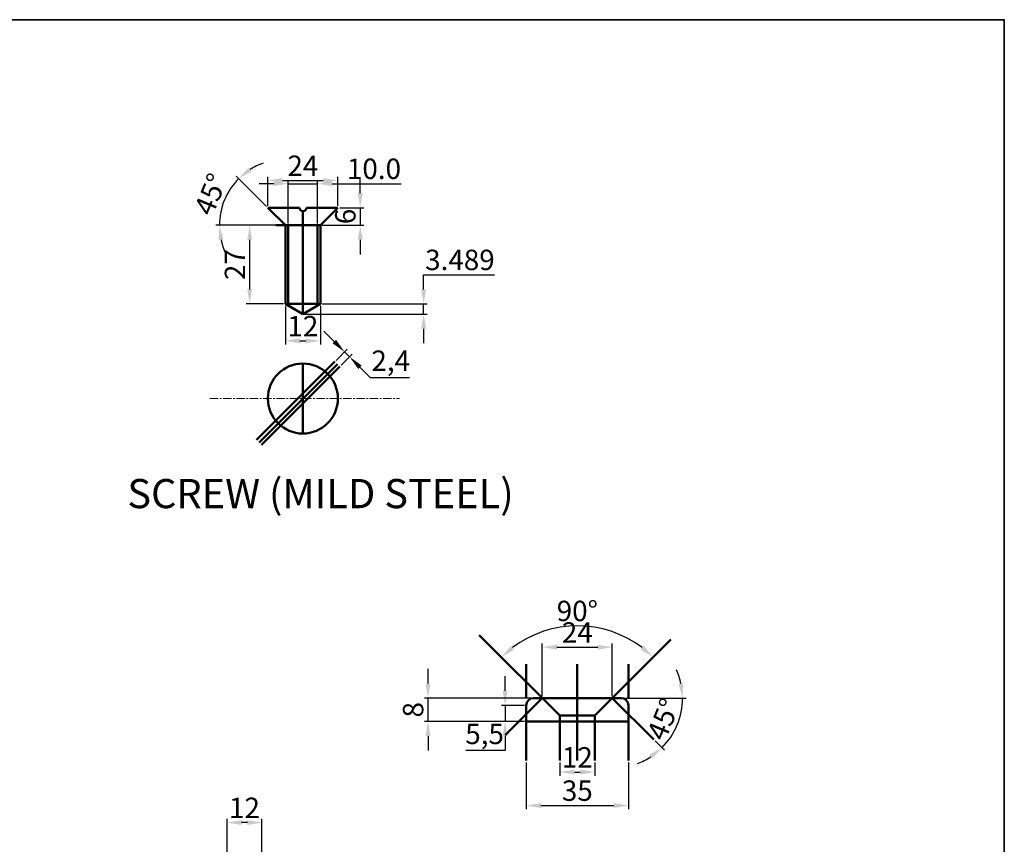
# Model space of a CAD drawing. Units: millimetres. Extents: x 4274 to 5106, y 2129 to 2785.
# Tile 4 of 4: x 4740 to 5077, y 2502 to 2785. Entities that reach past the tile are written whole.
import ezdxf

# ---------------------------------------------------------------- set-up
doc = ezdxf.new("R2010")
doc.units = ezdxf.units.MM
doc.header["$LTSCALE"] = 0.3
doc.linetypes.add('CENTER', pattern=[50.8, 31.75, -6.35, 6.35, -6.35])
for name, color, linetype, lineweight in [('M-CNTR', 1, 'CENTER', 18), ('M-DIMS', 2, 'Continuous', 25), ('M-OUTL', 7, 'Continuous', 50), ('M-TEXT', 3, 'Continuous', 25), ('M-TTLB', 7, 'Continuous', 35)]:
    doc.layers.add(name, color=color, linetype=linetype, lineweight=lineweight)
doc.styles.get("Standard").update_dxf_attribs({"font": 'arial.ttf'})
doc.dimstyles.new('ISO-25', dxfattribs={"dimtxt": 7, "dimasz": 5, "dimexe": 1.25, "dimexo": 0.625, "dimtad": 1, "dimtoh": 1, "dimtxsty": 'Standard', "dimcen": 2.5, "dimadec": 0, "dimazin": 0, "dimtfac": 1, "dimtmove": 0, "dimatfit": 3, "dimfxl": 1, "dimarcsym": 0})

# ---------------------------------------------------------------- blocks, each defined once
blk = doc.blocks.new('*D24')
at = {"layer": 'Defpoints', "color": 0, "ltscale": 0.3, "transparency": 16777216}
for p in [(4847.91, 2667.9), (4852.95, 2669.55), (4849.6, 2666.2)]:
    blk.add_point(p, dxfattribs=at)
at = {"layer": 'M-DIMS', "color": 0, "lineweight": -2, "ltscale": 0.3, "transparency": 16777216}
for p, q in [((4847.72, 2674.78), (4844.18, 2678.31)), ((4848.35, 2668.34), (4852.14, 2672.13)), ((4851.25, 2671.24), (4852.95, 2669.55)), ((4850.04, 2666.64), (4853.83, 2670.43)), ((4856.48, 2666.01), (4860.02, 2662.48)), ((4860.02, 2662.48), (4873.48, 2662.48))]:
    blk.add_line(p, q, dxfattribs=at)
at = {"layer": 'M-DIMS', "color": 0, "ltscale": 0.3, "transparency": 16777216}
for points in [[(4848.31, 2675.37), (4847.13, 2674.19), (4851.25, 2671.24)], [(4857.07, 2666.6), (4855.89, 2665.42), (4852.95, 2669.55)]]:
    blk.add_solid(points, dxfattribs=at)
at = {"layer": 'M-DIMS', "color": 0, "ltscale": 0.3, "transparency": 16777216, "insert": (4867.06, 2667.31), "char_height": 7, "attachment_point": 5}
blk.add_mtext('2,4', dxfattribs=at)
blk = doc.blocks.new('*D25')
at = {"layer": 'Defpoints', "color": 0, "ltscale": 0.3, "transparency": 16777216}
for p in [(4848.94, 2720.68), (4842.94, 2714.68), (4856.6, 2714.68)]:
    blk.add_point(p, dxfattribs=at)
at = {"layer": 'M-DIMS', "color": 0, "lineweight": -2, "ltscale": 0.3, "transparency": 16777216}
for p, q in [((4856.6, 2725.68), (4856.6, 2730.68)), ((4849.57, 2720.68), (4857.85, 2720.68)), ((4856.6, 2720.68), (4856.6, 2714.68)), ((4843.57, 2714.68), (4857.85, 2714.68)), ((4856.6, 2709.68), (4856.6, 2704.68))]:
    blk.add_line(p, q, dxfattribs=at)
at = {"layer": 'M-DIMS', "color": 0, "ltscale": 0.3, "transparency": 16777216}
for points in [[(4855.77, 2725.68), (4857.44, 2725.68), (4856.6, 2720.68)], [(4855.77, 2709.68), (4857.44, 2709.68), (4856.6, 2714.68)]]:
    blk.add_solid(points, dxfattribs=at)
at = {"layer": 'M-DIMS', "color": 0, "ltscale": 0.3, "transparency": 16777216, "insert": (4852.4, 2717.68), "char_height": 7, "attachment_point": 5, "rotation": 90}
blk.add_mtext('6', dxfattribs=at)
blk = doc.blocks.new('*D26')
at = {"layer": 'Defpoints', "color": 0, "ltscale": 0.3, "transparency": 16777216}
for p in [(4830.94, 2714.68), (4818.69, 2687.68), (4830.94, 2687.68)]:
    blk.add_point(p, dxfattribs=at)
at = {"layer": 'M-DIMS', "color": 0, "lineweight": -2, "ltscale": 0.3, "transparency": 16777216}
for p, q in [((4830.32, 2714.68), (4817.44, 2714.68)), ((4818.69, 2709.68), (4818.69, 2692.68)), ((4830.32, 2687.68), (4817.44, 2687.68))]:
    blk.add_line(p, q, dxfattribs=at)
at = {"layer": 'M-DIMS', "color": 0, "ltscale": 0.3, "transparency": 16777216}
for points in [[(4817.86, 2709.68), (4819.53, 2709.68), (4818.69, 2714.68)], [(4817.86, 2692.68), (4819.53, 2692.68), (4818.69, 2687.68)]]:
    blk.add_solid(points, dxfattribs=at)
at = {"layer": 'M-DIMS', "color": 0, "ltscale": 0.3, "transparency": 16777216, "insert": (4814.55, 2701.18), "char_height": 7, "attachment_point": 5, "rotation": 90}
blk.add_mtext('27', dxfattribs=at)
blk = doc.blocks.new('*D27')
at = {"layer": 'Defpoints', "color": 0, "ltscale": 0.3, "transparency": 16777216}
for p in [(4848.94, 2730.03), (4824.94, 2720.68), (4848.94, 2720.68)]:
    blk.add_point(p, dxfattribs=at)
at = {"layer": 'M-DIMS', "color": 0, "lineweight": -2, "ltscale": 0.3, "transparency": 16777216}
for p, q in [((4824.94, 2721.3), (4824.94, 2731.28)), ((4829.94, 2730.03), (4843.94, 2730.03)), ((4848.94, 2721.3), (4848.94, 2731.28))]:
    blk.add_line(p, q, dxfattribs=at)
at = {"layer": 'M-DIMS', "color": 0, "ltscale": 0.3, "transparency": 16777216}
for points in [[(4829.94, 2730.87), (4829.94, 2729.2), (4824.94, 2730.03)], [(4843.94, 2730.87), (4843.94, 2729.2), (4848.94, 2730.03)]]:
    blk.add_solid(points, dxfattribs=at)
at = {"layer": 'M-DIMS', "color": 0, "ltscale": 0.3, "transparency": 16777216, "insert": (4836.94, 2734.17), "char_height": 7, "attachment_point": 5}
blk.add_mtext('24', dxfattribs=at)
blk = doc.blocks.new('*D28')
at = {"layer": 'Defpoints', "color": 0, "ltscale": 0.3, "transparency": 16777216}
for p in [(4811.35, 2725.99), (4824.94, 2720.68), (4827.61, 2714.68), (4830.94, 2714.68), (4830.94, 2714.68)]:
    blk.add_point(p, dxfattribs=at)
at = {"layer": 'M-DIMS', "color": 0, "lineweight": -2, "ltscale": 0.3, "transparency": 16777216}
for p, q in [((4824.5, 2721.12), (4814.06, 2731.56)), ((4826.99, 2714.68), (4807.07, 2714.68))]:
    blk.add_line(p, q, dxfattribs=at)
for start, end in [(109.6287, 122.3144), (135, 180), (192.6856, 205.3713)]:
    blk.add_arc((4830.94, 2714.68), 22.63, start, end, dxfattribs=at)
at = {"layer": 'M-DIMS', "color": 0, "ltscale": 0.3, "transparency": 16777216}
for points in [[(4819.37, 2733.15), (4818.33, 2734.45), (4814.94, 2730.68)], [(4808.04, 2709.62), (4809.7, 2709.8), (4808.32, 2714.68)]]:
    blk.add_solid(points, dxfattribs=at)
at = {"layer": 'M-DIMS', "color": 0, "ltscale": 0.3, "transparency": 16777216, "insert": (4806.17, 2724.94), "char_height": 7, "attachment_point": 5, "rotation": 67.5}
blk.add_mtext('45°', dxfattribs=at)
blk = doc.blocks.new('*D29')
at = {"layer": 'Defpoints', "color": 0, "ltscale": 0.3, "transparency": 16777216}
for p in [(4830.94, 2687.68), (4842.94, 2687.68), (4842.94, 2675.03)]:
    blk.add_point(p, dxfattribs=at)
at = {"layer": 'M-DIMS', "color": 0, "lineweight": -2, "ltscale": 0.3, "transparency": 16777216}
for p, q in [((4830.94, 2687.05), (4830.94, 2673.78)), ((4842.94, 2687.05), (4842.94, 2673.78)), ((4835.94, 2675.03), (4837.94, 2675.03))]:
    blk.add_line(p, q, dxfattribs=at)
at = {"layer": 'M-DIMS', "color": 0, "ltscale": 0.3, "transparency": 16777216}
for points in [[(4835.94, 2675.87), (4835.94, 2674.2), (4830.94, 2675.03)], [(4837.94, 2675.87), (4837.94, 2674.2), (4842.94, 2675.03)]]:
    blk.add_solid(points, dxfattribs=at)
at = {"layer": 'M-DIMS', "color": 0, "ltscale": 0.3, "transparency": 16777216, "insert": (4836.94, 2679.17), "char_height": 7, "attachment_point": 5}
blk.add_mtext('12', dxfattribs=at)
blk = doc.blocks.new('*D34')
at = {"layer": 'Defpoints', "color": 0, "ltscale": 0.3, "transparency": 16777216}
for p in [(4810.92, 2509.83), (4810.92, 2495.1), (4822.92, 2495.1)]:
    blk.add_point(p, dxfattribs=at)
at = {"layer": 'M-DIMS', "color": 0, "lineweight": -2, "ltscale": 0.3, "transparency": 16777216}
for p, q in [((4810.92, 2495.72), (4810.92, 2511.08)), ((4817.92, 2509.83), (4815.92, 2509.83)), ((4822.92, 2495.72), (4822.92, 2511.08))]:
    blk.add_line(p, q, dxfattribs=at)
at = {"layer": 'M-DIMS', "color": 0, "ltscale": 0.3, "transparency": 16777216}
for points in [[(4815.92, 2510.66), (4815.92, 2508.99), (4810.92, 2509.83)], [(4817.92, 2510.66), (4817.92, 2508.99), (4822.92, 2509.83)]]:
    blk.add_solid(points, dxfattribs=at)
at = {"layer": 'M-DIMS', "color": 0, "ltscale": 0.3, "transparency": 16777216, "insert": (4816.92, 2513.97), "char_height": 7, "attachment_point": 5}
blk.add_mtext('12', dxfattribs=at)
blk = doc.blocks.new('*D35')
at = {"layer": 'Defpoints', "color": 0, "ltscale": 0.3, "transparency": 16777216}
for p in [(4897.41, 2574.14), (4940.56, 2576.03), (4963.15, 2572.62), (4925.04, 2546.51), (4937.04, 2546.51)]:
    blk.add_point(p, dxfattribs=at)
at = {"layer": 'M-DIMS', "color": 0, "lineweight": -2, "ltscale": 0.3, "transparency": 16777216}
blk.add_arc((4931.04, 2540.51), 36.78, 52.7961, 127.2039, dxfattribs=at)
at = {"layer": 'M-DIMS', "color": 0, "ltscale": 0.3, "transparency": 16777216}
for points in [[(4909.35, 2569.17), (4908.26, 2570.43), (4905.04, 2566.52)], [(4953.83, 2570.43), (4952.73, 2569.17), (4957.05, 2566.52)]]:
    blk.add_solid(points, dxfattribs=at)
at = {"layer": 'M-DIMS', "color": 0, "ltscale": 0.3, "transparency": 16777216, "insert": (4931.04, 2581.49), "char_height": 7, "attachment_point": 5}
blk.add_mtext('90°', dxfattribs=at)
blk = doc.blocks.new('*D36')
at = {"layer": 'Defpoints', "color": 0, "ltscale": 0.3, "transparency": 16777216}
for p in [(4943.04, 2569.97), (4919.04, 2552.51), (4943.04, 2552.51)]:
    blk.add_point(p, dxfattribs=at)
at = {"layer": 'M-DIMS', "color": 0, "lineweight": -2, "ltscale": 0.3, "transparency": 16777216}
for p, q in [((4919.04, 2553.14), (4919.04, 2571.22)), ((4924.04, 2569.97), (4938.04, 2569.97)), ((4943.04, 2553.14), (4943.04, 2571.22))]:
    blk.add_line(p, q, dxfattribs=at)
at = {"layer": 'M-DIMS', "color": 0, "ltscale": 0.3, "transparency": 16777216}
for points in [[(4924.04, 2570.8), (4924.04, 2569.14), (4919.04, 2569.97)], [(4938.04, 2570.8), (4938.04, 2569.14), (4943.04, 2569.97)]]:
    blk.add_solid(points, dxfattribs=at)
at = {"layer": 'M-DIMS', "color": 0, "ltscale": 0.3, "transparency": 16777216, "insert": (4931.04, 2574.11), "char_height": 7, "attachment_point": 5}
blk.add_mtext('24', dxfattribs=at)
blk = doc.blocks.new('*D37')
at = {"layer": 'Defpoints', "color": 0, "ltscale": 0.3, "transparency": 16777216}
for p in [(4916.04, 2552.51), (4943.04, 2552.51), (4946.04, 2552.51), (4963.88, 2540.48), (4957.25, 2538.31)]:
    blk.add_point(p, dxfattribs=at)
at = {"layer": 'M-DIMS', "color": 0, "lineweight": -2, "ltscale": 0.3, "transparency": 16777216}
for p, q in [((4946.67, 2552.51), (4968.35, 2552.51)), ((4957.69, 2537.86), (4960.94, 2534.62))]:
    blk.add_line(p, q, dxfattribs=at)
for start, end in [(11.9291, 23.8583), (315, 0), (291.1417, 303.0709)]:
    blk.add_arc((4943.04, 2552.51), 24.06, start, end, dxfattribs=at)
at = {"layer": 'M-DIMS', "color": 0, "ltscale": 0.3, "transparency": 16777216}
for points in [[(4967.41, 2557.57), (4965.75, 2557.4), (4967.1, 2552.51)], [(4955.65, 2533), (4956.7, 2531.7), (4960.05, 2535.5)]]:
    blk.add_solid(points, dxfattribs=at)
at = {"layer": 'M-DIMS', "color": 0, "ltscale": 0.3, "transparency": 16777216, "insert": (4961.4, 2544.91), "char_height": 7, "attachment_point": 5, "rotation": 67.5}
blk.add_mtext('45°', dxfattribs=at)
blk = doc.blocks.new('*D38')
at = {"layer": 'Defpoints', "color": 0, "ltscale": 0.3, "transparency": 16777216}
for p in [(4925.04, 2531.1), (4937.04, 2531.1), (4937.04, 2527.14)]:
    blk.add_point(p, dxfattribs=at)
at = {"layer": 'M-DIMS', "color": 0, "lineweight": -2, "ltscale": 0.3, "transparency": 16777216}
for p, q in [((4925.04, 2530.48), (4925.04, 2525.89)), ((4937.04, 2530.48), (4937.04, 2525.89)), ((4930.04, 2527.14), (4932.04, 2527.14))]:
    blk.add_line(p, q, dxfattribs=at)
at = {"layer": 'M-DIMS', "color": 0, "ltscale": 0.3, "transparency": 16777216}
for points in [[(4930.04, 2527.98), (4930.04, 2526.31), (4925.04, 2527.14)], [(4932.04, 2527.98), (4932.04, 2526.31), (4937.04, 2527.14)]]:
    blk.add_solid(points, dxfattribs=at)
at = {"layer": 'M-DIMS', "color": 0, "ltscale": 0.3, "transparency": 16777216, "insert": (4931.04, 2531.28), "char_height": 7, "attachment_point": 5}
blk.add_mtext('12', dxfattribs=at)
blk = doc.blocks.new('*D39')
at = {"layer": 'Defpoints', "color": 0, "ltscale": 0.3, "transparency": 16777216}
for p in [(4913.54, 2531.1), (4948.54, 2531.1), (4948.54, 2515.66)]:
    blk.add_point(p, dxfattribs=at)
at = {"layer": 'M-DIMS', "color": 0, "lineweight": -2, "ltscale": 0.3, "transparency": 16777216}
for p, q in [((4913.54, 2530.48), (4913.54, 2514.41)), ((4948.54, 2530.48), (4948.54, 2514.41)), ((4918.54, 2515.66), (4943.54, 2515.66))]:
    blk.add_line(p, q, dxfattribs=at)
at = {"layer": 'M-DIMS', "color": 0, "ltscale": 0.3, "transparency": 16777216}
for points in [[(4918.54, 2516.49), (4918.54, 2514.82), (4913.54, 2515.66)], [(4943.54, 2516.49), (4943.54, 2514.82), (4948.54, 2515.66)]]:
    blk.add_solid(points, dxfattribs=at)
at = {"layer": 'M-DIMS', "color": 0, "ltscale": 0.3, "transparency": 16777216, "insert": (4931.04, 2519.86), "char_height": 7, "attachment_point": 5}
blk.add_mtext('35', dxfattribs=at)
blk = doc.blocks.new('*D40')
at = {"layer": 'Defpoints', "color": 0, "ltscale": 0.3, "transparency": 16777216}
for p in [(4879.85, 2552.51), (4919.04, 2552.51), (4913.54, 2544.51)]:
    blk.add_point(p, dxfattribs=at)
at = {"layer": 'M-DIMS', "color": 0, "lineweight": -2, "ltscale": 0.3, "transparency": 16777216}
for p, q in [((4879.85, 2557.51), (4879.85, 2562.51)), ((4918.42, 2552.51), (4878.6, 2552.51)), ((4879.85, 2544.51), (4879.85, 2552.51)), ((4912.92, 2544.51), (4878.6, 2544.51)), ((4879.85, 2539.51), (4879.85, 2534.51))]:
    blk.add_line(p, q, dxfattribs=at)
at = {"layer": 'M-DIMS', "color": 0, "ltscale": 0.3, "transparency": 16777216}
for points in [[(4879.02, 2557.51), (4880.69, 2557.51), (4879.85, 2552.51)], [(4879.02, 2539.51), (4880.69, 2539.51), (4879.85, 2544.51)]]:
    blk.add_solid(points, dxfattribs=at)
at = {"layer": 'M-DIMS', "color": 0, "ltscale": 0.3, "transparency": 16777216, "insert": (4875.65, 2548.51), "char_height": 7, "attachment_point": 5, "rotation": 90}
blk.add_mtext('8', dxfattribs=at)
blk = doc.blocks.new('*D41')
at = {"layer": 'Defpoints', "color": 0, "ltscale": 0.3, "transparency": 16777216}
for p in [(4913.54, 2550.01), (4906.28, 2544.51), (4913.54, 2544.51)]:
    blk.add_point(p, dxfattribs=at)
at = {"layer": 'M-DIMS', "color": 0, "lineweight": -2, "ltscale": 0.3, "transparency": 16777216}
for p, q in [((4906.28, 2555.01), (4906.28, 2560.01)), ((4912.92, 2550.01), (4905.03, 2550.01)), ((4906.28, 2550.01), (4906.28, 2544.51)), ((4912.92, 2544.51), (4905.03, 2544.51)), ((4906.28, 2539.51), (4906.28, 2534.51)), ((4906.28, 2534.51), (4892.85, 2534.51))]:
    blk.add_line(p, q, dxfattribs=at)
at = {"layer": 'M-DIMS', "color": 0, "ltscale": 0.3, "transparency": 16777216}
for points in [[(4905.44, 2555.01), (4907.11, 2555.01), (4906.28, 2550.01)], [(4905.44, 2539.51), (4907.11, 2539.51), (4906.28, 2544.51)]]:
    blk.add_solid(points, dxfattribs=at)
at = {"layer": 'M-DIMS', "color": 0, "ltscale": 0.3, "transparency": 16777216, "insert": (4899.25, 2539.33), "char_height": 7, "attachment_point": 5}
blk.add_mtext('5,5', dxfattribs=at)
blk = doc.blocks.new('*D60')
at = {"layer": 'Defpoints', "color": 0, "ltscale": 0.3, "transparency": 16777216}
for p in [(4841.94, 2728.93), (4831.94, 2714.68), (4841.94, 2714.68)]:
    blk.add_point(p, dxfattribs=at)
at = {"layer": 'M-DIMS', "color": 0, "lineweight": -2, "ltscale": 0.3, "transparency": 16777216}
for p, q in [((4826.94, 2728.93), (4821.94, 2728.93)), ((4831.94, 2715.3), (4831.94, 2730.18)), ((4831.94, 2728.93), (4841.94, 2728.93)), ((4841.94, 2715.3), (4841.94, 2730.18)), ((4846.94, 2728.93), (4870.69, 2728.93))]:
    blk.add_line(p, q, dxfattribs=at)
at = {"layer": 'M-DIMS', "color": 0, "ltscale": 0.3, "transparency": 16777216}
for points in [[(4826.94, 2729.76), (4826.94, 2728.1), (4831.94, 2728.93)], [(4846.94, 2729.76), (4846.94, 2728.1), (4841.94, 2728.93)]]:
    blk.add_solid(points, dxfattribs=at)
at = {"layer": 'M-DIMS', "color": 0, "ltscale": 0.3, "transparency": 16777216, "insert": (4861.32, 2733.13), "char_height": 7, "attachment_point": 5}
blk.add_mtext('10.0', dxfattribs=at)
blk = doc.blocks.new('*D61')
at = {"layer": 'Defpoints', "color": 0, "ltscale": 0.3, "transparency": 16777216}
for p in [(4842.94, 2687.68), (4878.35, 2687.68), (4836.94, 2684.19)]:
    blk.add_point(p, dxfattribs=at)
at = {"layer": 'M-DIMS', "color": 0, "lineweight": -2, "ltscale": 0.3, "transparency": 16777216}
for p, q in [((4878.35, 2692.68), (4878.35, 2697.68)), ((4878.35, 2697.68), (4902.61, 2697.68)), ((4843.57, 2687.68), (4879.6, 2687.68)), ((4878.35, 2684.19), (4878.35, 2687.68)), ((4837.57, 2684.19), (4879.6, 2684.19)), ((4878.35, 2679.19), (4878.35, 2674.19))]:
    blk.add_line(p, q, dxfattribs=at)
at = {"layer": 'M-DIMS', "color": 0, "ltscale": 0.3, "transparency": 16777216}
for points in [[(4877.52, 2692.68), (4879.19, 2692.68), (4878.35, 2687.68)], [(4877.52, 2679.19), (4879.19, 2679.19), (4878.35, 2684.19)]]:
    blk.add_solid(points, dxfattribs=at)
at = {"layer": 'M-DIMS', "color": 0, "ltscale": 0.3, "transparency": 16777216, "insert": (4890.79, 2701.88), "char_height": 7, "attachment_point": 5}
blk.add_mtext('3.489', dxfattribs=at)

msp = doc.modelspace()

# ---------------------------------------------------------------- linework, layer by layer
at = {"layer": 'M-CNTR', "ltscale": 0.3}
msp.add_line((4805.0039, 2655.2403), (4870.1028, 2655.2403), dxfattribs=at)
at = {"layer": 'M-OUTL', "ltscale": 0.3}
for p, q in [((4824.9449, 2720.6786), (4835.7449, 2720.6786)), ((4830.9449, 2714.6786), (4824.9449, 2720.6786)), ((4836.9449, 2719.4786), (4836.9449, 2684.19)), ((4838.1449, 2720.6786), (4848.9449, 2720.6786)), ((4842.9449, 2714.6786), (4848.9449, 2720.6786)), ((4830.9449, 2714.6786), (4827.6113, 2714.6786)), ((4830.9449, 2714.6786), (4842.9449, 2714.6786)), ((4830.9449, 2714.6786), (4830.9449, 2687.6786)), ((4831.9449, 2714.6786), (4831.9449, 2687.6786)), ((4841.9449, 2714.6786), (4841.9449, 2687.6786)), ((4842.9449, 2714.6786), (4842.9449, 2687.6786)), ((4830.9449, 2687.6786), (4842.9449, 2687.6786)), ((4830.9449, 2687.6786), (4836.9449, 2684.19)), ((4836.9449, 2684.19), (4842.9449, 2687.6786)), ((4847.9054, 2667.8979), (4821.0489, 2641.0414)), ((4848.7539, 2667.0493), (4821.8974, 2640.1929)), ((4849.6024, 2666.2008), (4822.746, 2639.3444)), ((4836.9449, 2667.2403), (4836.9449, 2643.2403)), ((4925.0423, 2546.5113), (4897.4126, 2574.1411)), ((4937.0423, 2546.5113), (4963.1532, 2572.6221)), ((4913.5423, 2564.1465), (4913.5423, 2552.5113)), ((4931.0423, 2564.1465), (4931.0423, 2531.1046)), ((4948.5423, 2564.1465), (4948.5423, 2552.5113)), ((4919.0423, 2552.5113), (4906.2751, 2539.744)), ((4916.0423, 2552.5113), (4946.0423, 2552.5113)), ((4943.0423, 2552.5113), (4957.2482, 2538.3054)), ((4913.5423, 2550.0113), (4913.5423, 2531.1046)), ((4948.5423, 2550.0113), (4948.5423, 2531.1046)), ((4925.0423, 2546.5113), (4925.0423, 2531.1046)), ((4925.0423, 2546.5113), (4937.0423, 2546.5113)), ((4937.0423, 2546.5113), (4937.0423, 2531.1046)), ((4913.5423, 2544.5113), (4948.5423, 2544.5113))]:
    msp.add_line(p, q, dxfattribs=at)
msp.add_circle((4836.9449, 2655.2403), 12, dxfattribs=at)
for centre, radius, start, end in [((4836.9449, 2720.6786), 1.2, 180, 0), ((4916.0423, 2550.0113), 2.5, 90, 180), ((4946.0423, 2550.0113), 2.5, 0, 90)]:
    msp.add_arc(centre, radius, start, end, dxfattribs=at)
at = {"layer": 'M-TTLB', "ltscale": 0.3}
msp.add_lwpolyline([(5077.4601, 2139.9092), (4273.9655, 2139.9092), (4273.9655, 2785.1666), (5077.4601, 2785.1666)], close=True, dxfattribs=at)

# ---------------------------------------------------------------- texts
at = {"layer": 'M-TEXT', "ltscale": 0.3, "insert": (4776.7392, 2627.6432), "char_height": 10, "attachment_point": 1}
msp.add_mtext_dynamic_manual_height_columns('SCREW (MILD STEEL)', width=160.066883, gutter_width=12.5, heights=[0], dxfattribs=at)

# ---------------------------------------------------------------- dimensions: what is measured, and where the dimension line sits
at = {"layer": 'M-DIMS', "ltscale": 0.3}
for base, p1, p2, override, picture, middle in [((4848.9449, 2730.0332), (4824.9449, 2720.6786), (4848.9449, 2720.6786), {"dimclrd": 0, "dimclre": 0, "dimclrt": 0}, '*D27', (4836.9449, 2734.1725)), ((4841.9449, 2728.9286), (4831.9449, 2714.6786), (4841.9449, 2714.6786), {"dimdec": 1, "dimlfac": 1, "dimrnd": 0, "dimzin": 0, "dimdsep": 46, "dimlunit": 2}, '*D60', (4861.3199, 2733.1277)), ((4842.9449, 2675.0319), (4830.9449, 2687.6786), (4842.9449, 2687.6786), {"dimclrd": 0, "dimclre": 0, "dimclrt": 0}, '*D29', (4836.9449, 2679.1712)), ((4943.0423, 2569.9705), (4919.0423, 2552.5113), (4943.0423, 2552.5113), {"dimclrd": 0, "dimclre": 0, "dimclrt": 0}, '*D36', (4931.0423, 2574.1099)), ((4937.0423, 2527.1439), (4925.0423, 2531.1046), (4937.0423, 2531.1046), {"dimclrd": 0, "dimclre": 0, "dimclrt": 0}, '*D38', (4931.0423, 2531.2832)), ((4948.5423, 2515.6567), (4913.5423, 2531.1046), (4948.5423, 2531.1046), {"dimclrd": 0, "dimclre": 0, "dimclrt": 0}, '*D39', (4931.0423, 2519.8581)), ((4810.9214, 2509.8264), (4822.9214, 2495.0953), (4810.9214, 2495.0953), {"dimclrd": 0, "dimclre": 0, "dimclrt": 0}, '*D34', (4816.9214, 2513.9657))]:
    dim = msp.add_linear_dim(base=base, p1=p1, p2=p2, dimstyle='ISO-25', override=override, dxfattribs=at)
    dim.commit()
    dim.dimension.update_dxf_attribs({"geometry": picture, "text_midpoint": middle})
for base, line1, line2, picture, middle in [((4811.3475, 2725.9932), ((4830.9449, 2714.6786), (4827.6113, 2714.6786)), ((4830.9449, 2714.6786), (4824.9449, 2720.6786)), '*D28', (4806.1721, 2724.9399)), ((4940.5604, 2576.0332), ((4937.0423, 2546.5113), (4963.1532, 2572.6221)), ((4925.0423, 2546.5113), (4897.4126, 2574.1411)), '*D35', (4931.0423, 2581.4853)), ((4963.8776, 2540.482), ((4916.0423, 2552.5113), (4946.0423, 2552.5113)), ((4943.0423, 2552.5113), (4957.2482, 2538.3054)), '*D37', (4961.4033, 2544.9059))]:
    dim = msp.add_angular_dim_2l(base=base, line1=line1, line2=line2, dimstyle='ISO-25', override={"dimclrd": 0, "dimclre": 0, "dimclrt": 0}, dxfattribs=at)
    dim.commit()
    dim.dimension.update_dxf_attribs({"geometry": picture, "text_midpoint": middle})
for base, p1, p2, override, picture, middle in [((4856.6022, 2714.6786), (4848.9449, 2720.6786), (4842.9449, 2714.6786), {"dimclrd": 0, "dimclre": 0, "dimclrt": 0}, '*D25', (4852.4032, 2717.6786)), ((4818.6924, 2687.6786), (4830.9449, 2714.6786), (4830.9449, 2687.6786), {"dimclrd": 0, "dimclre": 0, "dimclrt": 0}, '*D26', (4814.5531, 2701.1786)), ((4878.3528, 2687.6786), (4836.9449, 2684.19), (4842.9449, 2687.6786), {"dimdec": 3, "dimlfac": 1, "dimrnd": 0, "dimzin": 0, "dimdsep": 46, "dimlunit": 2}, '*D61', (4890.7933, 2701.88)), ((4906.2751, 2544.5113), (4913.5423, 2550.0113), (4913.5423, 2544.5113), {"dimclrd": 0, "dimclre": 0, "dimclrt": 0}, '*D41', (4899.2517, 2539.3287))]:
    dim = msp.add_linear_dim(base=base, p1=p1, p2=p2, angle=90, dimstyle='ISO-25', override=override, dxfattribs=at)
    dim.commit()
    dim.dimension.update_dxf_attribs({"geometry": picture, "text_midpoint": middle})
dim = msp.add_aligned_dim(p1=(4847.9054, 2667.8979), p2=(4849.6024, 2666.2008), distance=4.7319, dimstyle='ISO-25', override={"dimclrd": 0, "dimclre": 0, "dimclrt": 0}, dxfattribs=at)
dim.commit()
dim.dimension.update_dxf_attribs({"geometry": '*D24', "text_midpoint": (4867.0619, 2667.3074)})
dim = msp.add_linear_dim(base=(4879.8526, 2552.5113), p1=(4913.5423, 2544.5113), p2=(4919.0423, 2552.5113), angle=90, dimstyle='ISO-25', override={"dimclrd": 0, "dimclre": 0, "dimclrt": 0}, dxfattribs=at)
dim.commit()
dim.dimension.update_dxf_attribs({"geometry": '*D40', "text_midpoint": (4879.8526, 2548.5113), "dimtype": 160})

doc.saveas('drawing.dxf')
